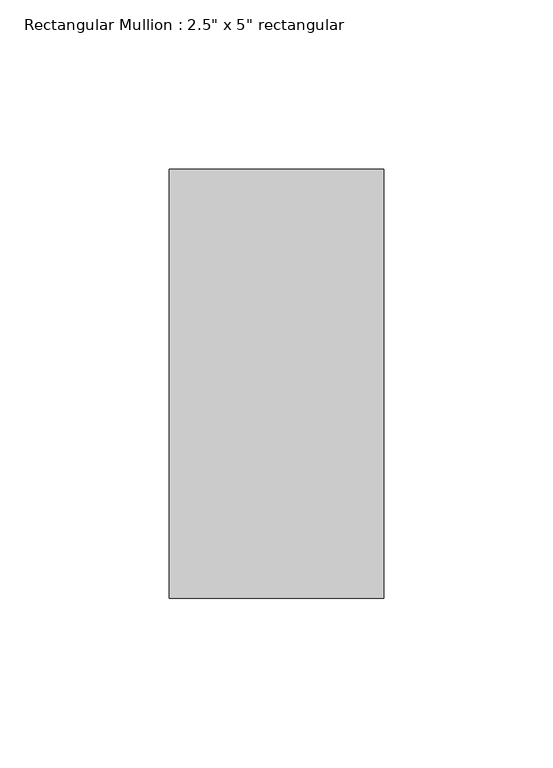
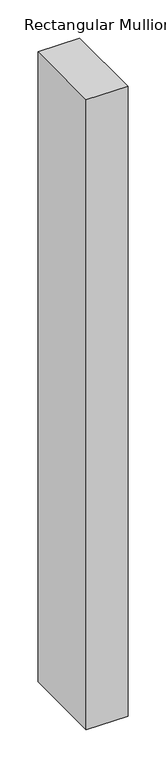
"""IFC4 building model written with IfcOpenShell, lengths in millimetres: member geometry."""

from ifc_helpers import new_model, si_unit, frame, origin, place, context, project, spatial, polyline, outline, extrude, source, transform, mapped, element, save


def member_8346ef35(model_context):
    return source(origin(), model_context, "Body", "SweptSolid", [
        extrude(outline(polyline([(0.0, 63.5), (0.0, -63.5), (-63.5, -63.5), (-63.5, 63.5), (0.0, 63.5)])), frame((0.0, 0.0, -1009.9541688), z_axis=(0.0, 0.0, 1.0), x_axis=(1.0, 0.0, 0.0)), (0.0, 0.0, 1.0), 1009.9541688),
    ])


if __name__ == "__main__":
    model = new_model("IFC4")
    model_context = context("Model", 3, world=origin())
    ifc_project = project(units=[si_unit("LENGTHUNIT", "METRE", prefix="MILLI")], contexts=[model_context])
    site = spatial("IfcSite", under=ifc_project)
    building = spatial("IfcBuilding", under=site)
    placement = place(None, origin())
    member_shape = member_8346ef35(model_context)
    element("IfcMember", 1, ObjectType="Rectangular Mullion : 2.5\" x 5\" rectangular", at=placement, inside=building, context=model_context, shape_type="MappedRepresentation", body=[
        mapped(member_shape, transform((0.0, 0.0, 0.0), x_axis=(1.0, 0.0, 0.0), y_axis=(0.0, 1.0, 0.0), z_axis=(0.0, 0.0, 1.0))),
    ])
    save(model, "model.ifc")

# Revit data of these elements
# Type "Rectangular Mullion : 2.5\" x 5\" rectangular"
#   built-in parameter 1007304 = 0.416667 (stored number, unit not read)
#   built-in parameter 1007301 = 0.104167 (stored number, unit not read)
#   built-in parameter 1007300 = 0.104167 (stored number, unit not read)
# Element 1 (IfcMember, "Rectangular Mullion : 2.5\" x 5\" rectangular")
#   Materials on its faces: "Aluminum"
# Materials
#   "Aluminum": class "Metal", colour RGB 247 247 247, transparency 0, Description = "Aluminum 6061", Cost = 0
